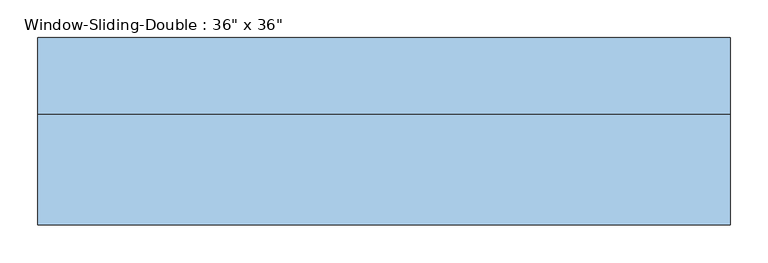
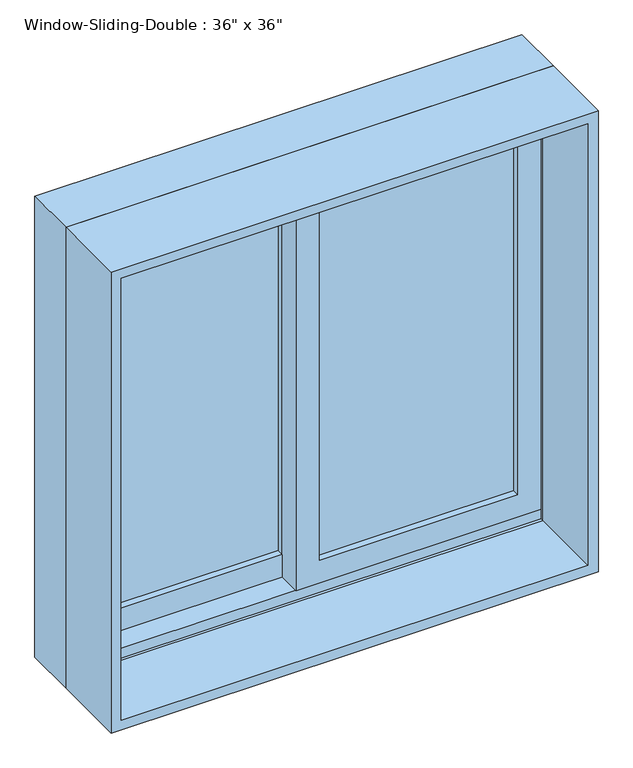
"""IFC4 building model written with IfcOpenShell, lengths in millimetres: window geometry."""

from ifc_helpers import new_model, si_unit, frame, origin, place, context, project, spatial, polyline, outline, extrude, faceted_brep, source, transform, mapped, element, save


def window_3ee5ce78(model_context):
    return source(origin(), model_context, "Body", "SolidModel", [
        extrude(outline(polyline([(952.5, 438.15), (1809.75, 438.15), (1809.75, -22.225), (952.5, -22.225), (952.5, 438.15)]), holes=[polyline([(996.95, 22.225), (1765.3, 22.225), (1765.3, 393.7), (996.95, 393.7), (996.95, 22.225)])]), frame((0.0, 34.29, 0.0), z_axis=(0.0, 1.0, 0.0), x_axis=(0.0, 0.0, 1.0)), (0.0, 0.0, 1.0), 44.45),
        extrude(outline(polyline([(933.45, -438.15), (933.45, 22.225), (1809.75, 22.225), (1809.75, -438.15), (933.45, -438.15)]), holes=[polyline([(1765.3, -22.225), (996.95, -22.225), (996.95, -393.7), (1765.3, -393.7), (1765.3, -22.225)])]), frame((0.0, 78.74, 0.0), z_axis=(0.0, 1.0, 0.0), x_axis=(0.0, 0.0, 1.0)), (0.0, 0.0, 1.0), 44.45),
        extrude(outline(polyline([(-22.225, 110.49), (-22.225, 104.14), (-393.7, 104.14), (-393.7, 110.49), (-22.225, 110.49)])), frame((0.0, 0.0, 996.95), z_axis=(0.0, 0.0, 1.0), x_axis=(1.0, 0.0, 0.0)), (0.0, 0.0, 1.0), 768.35),
        extrude(outline(polyline([(-22.225, 97.79), (-22.225, 91.44), (-393.7, 91.44), (-393.7, 97.79), (-22.225, 97.79)])), frame((0.0, 0.0, 996.95), z_axis=(0.0, 0.0, 1.0), x_axis=(1.0, 0.0, 0.0)), (0.0, 0.0, 1.0), 768.35),
        extrude(outline(polyline([(393.7, 66.04), (393.7, 59.69), (22.225, 59.69), (22.225, 66.04), (393.7, 66.04)])), frame((0.0, 0.0, 996.95), z_axis=(0.0, 0.0, 1.0), x_axis=(1.0, 0.0, 0.0)), (0.0, 0.0, 1.0), 768.35),
        extrude(outline(polyline([(393.7, 53.34), (393.7, 46.99), (22.225, 46.99), (22.225, 53.34), (393.7, 53.34)])), frame((0.0, 0.0, 996.95), z_axis=(0.0, 0.0, 1.0), x_axis=(1.0, 0.0, 0.0)), (0.0, 0.0, 1.0), 768.35),
        extrude(outline(polyline([(1828.8, -457.2), (914.4, -457.2), (914.4, 457.2), (1828.8, 457.2), (1828.8, -457.2)]), holes=[polyline([(1809.75, 438.15), (933.45, 438.15), (933.45, -438.15), (1809.75, -438.15), (1809.75, 438.15)])]), frame((0.0, -118.11, 0.0), z_axis=(0.0, 1.0, 0.0), x_axis=(0.0, 0.0, 1.0)), (0.0, 0.0, 1.0), 146.05),
        faceted_brep([(-457.2, 27.94, 914.4), (-457.2, 129.54, 914.4), (457.2, 129.54, 914.4), (457.2, 27.94, 914.4), (-416.2778905, 129.54, 1787.8778905), (-416.2778905, 123.19, 1787.8778905), (-416.2778905, 123.19, 933.45), (-416.2778905, 129.54, 933.45), (416.2778905, 123.19, 1787.8778905), (416.2778905, 123.19, 933.45), (438.15, 123.19, 933.45), (438.15, 123.19, 1809.75), (-438.15, 123.19, 1809.75), (-438.15, 123.19, 933.45), (-438.15, 27.94, 1809.75), (-438.15, 27.94, 933.45), (-438.15, 34.29, 933.45), (-438.15, 34.29, 952.5), (-438.15, 78.74, 952.5), (-438.15, 78.74, 933.45), (457.2, 27.94, 1828.8), (-457.2, 27.94, 1828.8), (438.15, 27.94, 1809.75), (438.15, 27.94, 933.45), (-457.2, 129.54, 1828.8), (457.2, 129.54, 1828.8), (416.2778905, 129.54, 933.45), (416.2778905, 129.54, 1787.8778905), (438.15, 78.74, 933.45), (438.15, 78.74, 952.5), (438.15, 34.29, 952.5), (438.15, 34.29, 933.45)], [[[0, 1, 2, 3]], [[4, 5, 6, 7]], [[5, 8, 9, 10, 11, 12, 13, 6]], [[12, 14, 15, 16, 17, 18, 19, 13]], [[0, 3, 20, 21], [22, 23, 15, 14]], [[24, 1, 0, 21]], [[2, 1, 24, 25], [4, 7, 26, 27]], [[5, 4, 27, 8]], [[12, 11, 22, 14]], [[21, 20, 25, 24]], [[8, 27, 26, 9]], [[22, 11, 10, 28, 29, 30, 31, 23]], [[20, 3, 2, 25]], [[26, 7, 6, 13, 19, 28, 10, 9]], [[28, 19, 18, 29]], [[29, 18, 17, 30]], [[30, 17, 16, 31]], [[15, 23, 31, 16]]]),
    ])


if __name__ == "__main__":
    model = new_model("IFC4")
    model_context = context("Model", 3, world=origin())
    ifc_project = project(units=[si_unit("LENGTHUNIT", "METRE", prefix="MILLI")], contexts=[model_context])
    site = spatial("IfcSite", under=ifc_project)
    building = spatial("IfcBuilding", under=site)
    placement = place(None, origin())
    window_shape = window_3ee5ce78(model_context)
    element("IfcWindow", 1, ObjectType="Window-Sliding-Double : 36\" x 36\"", at=placement, inside=building, context=model_context, shape_type="MappedRepresentation", body=[
        mapped(window_shape, transform((0.0, 0.0, 0.0), x_axis=(1.0, 0.0, 0.0), y_axis=(0.0, 1.0, 0.0), z_axis=(0.0, 0.0, 1.0))),
    ])
    save(model, "model.ifc")

# Revit data of these elements
# Type "Window-Sliding-Double : 36\" x 36\""
#   Type Mark = "51"
#   Fire Rating = "0.5h"
#   Assembly Code = "B2020100"
#   Analytic Construction = "Double glazing - domestic"
#   Window Inset [instance default] = 0' - 0"
#   Wall Thickness [instance default] = 0' - 6"
#   Visual Light Transmittance = 0.81
#   Thermal Resistance (R) = 0.319569 (m²·K)/W
#   Solar Heat Gain Coefficient = 0.76
#   Muntin Width = 1' - 2 5/8"
#   Muntin Height = 2' - 6 1/4"
#   Interior Wall Closure [instance default] = 0' - 2 3/4"
#   Heat Transfer Coefficient (U) = 3.12929 W/(m²·K)
#   Frame Extension [instance default] = 0' - 0 1/4"
#   Exterior Wall Closure [instance default] = 0' - 1 1/4"
#   Rough Width = 3' - 0 1/2"
#   Rough Height = 3' - 0 1/2"
#   Height = 3' - 0"
#   Extension Jamb [instance default] = 0' - 2 3/4"
#   Default Sill Height = 3' - 0"
#   Width = 3' - 0"
#   Interior Trim Visibility [instance default] = yes
#   Indicator Visibility [instance default] = yes
#   Exterior Trim Visibility [instance default] = yes
#   Muntin Visibility = yes
#   Extension Jamb Visibility [instance default] = yes
#   Muntin Pattern = Muntin Pattern_2x2 : Muntin Pattern_2x2
#   Interior Trim Material = Wood - Stained
#   Interior Trim = Trim-Window-Interior-Flat : Picture Frame
#   Interior Frame Material = Wood - Stained
#   Glass Panel Material = Glass
#   Exterior Trim Material = Clad - White
#   Exterior Trim = Trim-Window-Exterior-Flat : with Sill
#   Exterior Frame Material = Clad - White
#   Wall Closure = (empty or 0)
# Element 1 (IfcWindow, "Window-Sliding-Double : 36\" x 36\"")
#   Wall Thickness = 0' - 9"
#   Extension Jamb = 0' - 5 3/4"
#   Materials on its faces: "Wood - Stained", "Glass", "Clad - White"
# Materials
#   "Wood - Stained": class "Wood", colour RGB 227 170 128, transparency 0, Cost = 0
#   "Glass": class "Glass", colour RGB 0 128 192, transparency 0.9, Description = "Soda Lime Glass", Cost = 0
#   "Clad - White": class "Wood", colour RGB 242 242 238, transparency 0, Cost = 0
